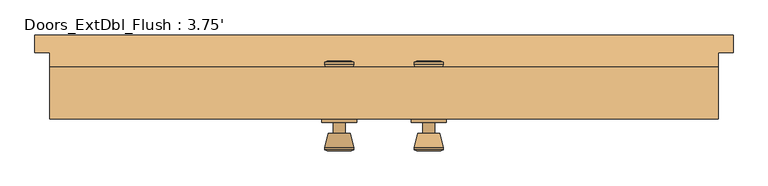
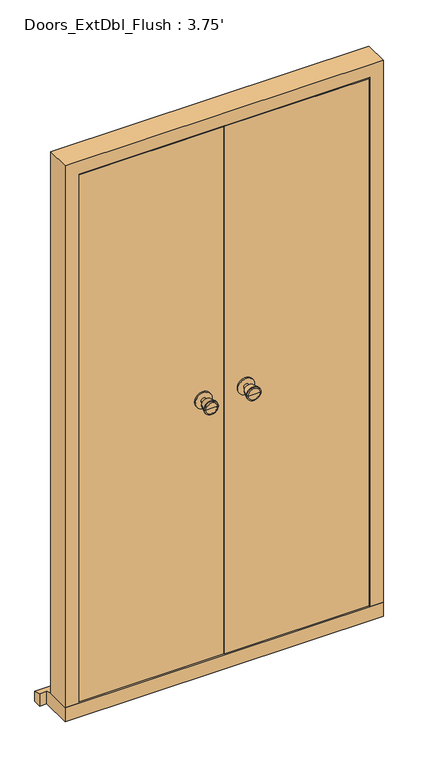
"""IFC4 building model written with IfcOpenShell, lengths in millimetres: door geometry, Doors_ExtDbl_Flush : 3.75'."""

from ifc_helpers import new_model, si_unit, point, frame, frame_2d, origin, place, context, project, spatial, polyline, circle_curve, trimmed, segment, composite_curve, outline, extrude, faceted_brep, source, transform, mapped, element, save
from ifc_brep_helpers import plane_surface, cylinder_surface, revolved_surface, advanced_brep


def doors_extdbl_flush_3_75_39ca422f(model_context):
    return source(origin(), model_context, "Body", "SolidModel", [
        advanced_brep(
        [(-76.5, -43.8, 1050.0), (-66.5, -43.8, 1050.0), (-86.5, -43.8, 1050.0), (-96.9758676, -92.8, 1050.0), (-56.0241324, -92.8, 1050.0), (-76.5, -92.8, 1050.0), (-101.5, -90.9721319, 1050.0), (-51.5, -90.9721319, 1050.0), (-101.5, -87.5084537, 1050.0), (-51.5, -87.5084537, 1050.0), (-95.136236, -62.8, 1050.0), (-57.863764, -62.8, 1050.0), (-86.5, -62.8, 1050.0), (-66.5, -62.8, 1050.0)],
        [
            (0, 1),
            (1, 2, circle_curve(frame((-76.5, -43.8, 1050.0), z_axis=(0.0, 1.0, 0.0), x_axis=(1.0, 0.0, 0.0)), 10.0)),
            (2, 0),
            (2, 1, circle_curve(frame((-76.5, -43.8, 1050.0), z_axis=(0.0, 1.0, 0.0), x_axis=(1.0, 0.0, 0.0)), 10.0)),
            (3, 4, circle_curve(frame((-76.5, -92.8, 1050.0), z_axis=(0.0, -1.0, 0.0), x_axis=(1.0, 0.0, 0.0)), 20.4758676)),
            (4, 5),
            (5, 3),
            (4, 3, circle_curve(frame((-76.5, -92.8, 1050.0), z_axis=(0.0, -1.0, 0.0), x_axis=(1.0, 0.0, 0.0)), 20.4758676)),
            (6, 7, circle_curve(frame((-76.5, -90.9721319, 1050.0), z_axis=(0.0, -1.0, 0.0), x_axis=(1.0, 0.0, 0.0)), 25.0)),
            (7, 4),
            (3, 6),
            (7, 6, circle_curve(frame((-76.5, -90.9721319, 1050.0), z_axis=(0.0, -1.0, 0.0), x_axis=(1.0, 0.0, 0.0)), 25.0)),
            (8, 9, circle_curve(frame((-76.5, -87.5084537, 1050.0), z_axis=(0.0, -1.0, 0.0), x_axis=(1.0, 0.0, 0.0)), 25.0)),
            (9, 7),
            (6, 8),
            (9, 8, circle_curve(frame((-76.5, -87.5084537, 1050.0), z_axis=(0.0, -1.0, 0.0), x_axis=(1.0, 0.0, 0.0)), 25.0)),
            (10, 11, circle_curve(frame((-76.5, -62.8, 1050.0), z_axis=(0.0, -1.0, 0.0), x_axis=(1.0, 0.0, 0.0)), 18.636236)),
            (11, 9),
            (8, 10),
            (11, 10, circle_curve(frame((-76.5, -62.8, 1050.0), z_axis=(0.0, -1.0, 0.0), x_axis=(1.0, 0.0, 0.0)), 18.636236)),
            (12, 13, circle_curve(frame((-76.5, -62.8, 1050.0), z_axis=(0.0, -1.0, 0.0), x_axis=(1.0, 0.0, 0.0)), 10.0)),
            (13, 11),
            (10, 12),
            (13, 12, circle_curve(frame((-76.5, -62.8, 1050.0), z_axis=(0.0, -1.0, 0.0), x_axis=(1.0, 0.0, 0.0)), 10.0)),
            (1, 13),
            (12, 2),
        ],
        [
            plane_surface(frame((-76.5, -43.8, 1050.0), z_axis=(0.0, 1.0, 0.0), x_axis=(1.0, 0.0, 0.0))),
            plane_surface(frame((-76.5, -92.8, 1050.0), z_axis=(0.0, -1.0, 0.0), x_axis=(1.0, 0.0, 0.0))),
            revolved_surface(polyline([(-56.0241324, -92.8, 1050.0), (-51.5, -90.9721319, 1050.0)]), (-76.5, -43.8, 1050.0), (0.0, 1.0, 0.0)),
            cylinder_surface(frame((-76.5, -43.8, 1050.0), z_axis=(0.0, 1.0, 0.0), x_axis=(1.0, 0.0, 0.0)), 25.0),
            revolved_surface(polyline([(-51.5, -87.5084537, 1050.0), (-57.863764, -62.8, 1050.0)]), (-76.5, -43.8, 1050.0), (0.0, 1.0, 0.0)),
            plane_surface(frame((-76.5, -62.8, 1050.0), z_axis=(0.0, 1.0, 0.0), x_axis=(1.0, 0.0, 0.0))),
            cylinder_surface(frame((-76.5, -43.8, 1050.0), z_axis=(0.0, 1.0, 0.0), x_axis=(1.0, 0.0, 0.0)), 10.0),
        ],
        [
            (0, [[1, 2, 3]]),
            (0, [[-3, 4, -1]]),
            (1, [[5, 6, 7]]),
            (1, [[8, -7, -6]]),
            (2, [[9, 10, -5, 11]]),
            (2, [[12, -11, -8, -10]]),
            (3, [[13, 14, -9, 15]]),
            (3, [[16, -15, -12, -14]]),
            (4, [[17, 18, -13, 19]]),
            (4, [[20, -19, -16, -18]]),
            (5, [[21, 22, -17, 23]]),
            (5, [[24, -23, -20, -22]]),
            (6, [[-2, 25, -21, 26]]),
            (6, [[-4, -26, -24, -25]]),
        ],
    ),
        extrude(outline(composite_curve([segment(trimmed(circle_curve(frame_2d((1050.0, -76.5)), 30.0), [point((1050.0, -46.5))], [point((1050.0, -106.5))], False, "CARTESIAN"), True, "CONTINUOUS"), segment(trimmed(circle_curve(frame_2d((1050.0, -76.5)), 30.0), [point((1050.0, -106.5))], [point((1050.0, -46.5))], False, "CARTESIAN"), True, "CONTINUOUS")], self_intersect=False)), frame((0.0, -43.8, 0.0), z_axis=(0.0, 1.0, 0.0), x_axis=(0.0, 0.0, 1.0)), (0.0, 0.0, 1.0), 6.0),
        advanced_brep(
        [(-76.5, 12.2, 1050.0), (-86.5, 12.2, 1050.0), (-66.5, 12.2, 1050.0), (-96.9758676, 61.2, 1050.0), (-76.5, 61.2, 1050.0), (-56.0241324, 61.2, 1050.0), (-101.5, 59.3721319, 1050.0), (-51.5, 59.3721319, 1050.0), (-101.5, 55.9084537, 1050.0), (-51.5, 55.9084537, 1050.0), (-95.136236, 31.2, 1050.0), (-57.863764, 31.2, 1050.0), (-86.5, 31.2, 1050.0), (-66.5, 31.2, 1050.0)],
        [
            (0, 1),
            (1, 2, circle_curve(frame((-76.5, 12.2, 1050.0), z_axis=(0.0, -1.0, 0.0), x_axis=(1.0, 0.0, 0.0)), 10.0)),
            (2, 0),
            (2, 1, circle_curve(frame((-76.5, 12.2, 1050.0), z_axis=(0.0, -1.0, 0.0), x_axis=(1.0, 0.0, 0.0)), 10.0)),
            (3, 4),
            (4, 5),
            (5, 3, circle_curve(frame((-76.5, 61.2, 1050.0), z_axis=(0.0, 1.0, 0.0), x_axis=(1.0, 0.0, 0.0)), 20.4758676)),
            (3, 5, circle_curve(frame((-76.5, 61.2, 1050.0), z_axis=(0.0, 1.0, 0.0), x_axis=(1.0, 0.0, 0.0)), 20.4758676)),
            (6, 3),
            (5, 7),
            (7, 6, circle_curve(frame((-76.5, 59.3721319, 1050.0), z_axis=(0.0, 1.0, 0.0), x_axis=(1.0, 0.0, 0.0)), 25.0)),
            (6, 7, circle_curve(frame((-76.5, 59.3721319, 1050.0), z_axis=(0.0, 1.0, 0.0), x_axis=(1.0, 0.0, 0.0)), 25.0)),
            (8, 6),
            (7, 9),
            (9, 8, circle_curve(frame((-76.5, 55.9084537, 1050.0), z_axis=(0.0, 1.0, 0.0), x_axis=(1.0, 0.0, 0.0)), 25.0)),
            (8, 9, circle_curve(frame((-76.5, 55.9084537, 1050.0), z_axis=(0.0, 1.0, 0.0), x_axis=(1.0, 0.0, 0.0)), 25.0)),
            (10, 8),
            (9, 11),
            (11, 10, circle_curve(frame((-76.5, 31.2, 1050.0), z_axis=(0.0, 1.0, 0.0), x_axis=(1.0, 0.0, 0.0)), 18.636236)),
            (10, 11, circle_curve(frame((-76.5, 31.2, 1050.0), z_axis=(0.0, 1.0, 0.0), x_axis=(1.0, 0.0, 0.0)), 18.636236)),
            (12, 10),
            (11, 13),
            (13, 12, circle_curve(frame((-76.5, 31.2, 1050.0), z_axis=(0.0, 1.0, 0.0), x_axis=(1.0, 0.0, 0.0)), 10.0)),
            (12, 13, circle_curve(frame((-76.5, 31.2, 1050.0), z_axis=(0.0, 1.0, 0.0), x_axis=(1.0, 0.0, 0.0)), 10.0)),
            (1, 12),
            (13, 2),
        ],
        [
            plane_surface(frame((-76.5, 12.2, 1050.0), z_axis=(0.0, -1.0, 0.0), x_axis=(1.0, 0.0, 0.0))),
            plane_surface(frame((-76.5, 61.2, 1050.0), z_axis=(0.0, 1.0, 0.0), x_axis=(1.0, 0.0, 0.0))),
            revolved_surface(polyline([(-56.0241324, 61.2, 1050.0), (-51.5, 59.3721319, 1050.0)]), (-76.5, 12.2, 1050.0), (0.0, -1.0, 0.0)),
            cylinder_surface(frame((-76.5, 12.2, 1050.0), z_axis=(0.0, -1.0, 0.0), x_axis=(1.0, 0.0, 0.0)), 25.0),
            revolved_surface(polyline([(-51.5, 55.9084537, 1050.0), (-57.863764, 31.2, 1050.0)]), (-76.5, 12.2, 1050.0), (0.0, -1.0, 0.0)),
            plane_surface(frame((-76.5, 31.2, 1050.0), z_axis=(0.0, -1.0, 0.0), x_axis=(1.0, 0.0, 0.0))),
            cylinder_surface(frame((-76.5, 12.2, 1050.0), z_axis=(0.0, -1.0, 0.0), x_axis=(1.0, 0.0, 0.0)), 10.0),
        ],
        [
            (0, [[1, 2, 3]]),
            (0, [[-3, 4, -1]]),
            (1, [[5, 6, 7]]),
            (1, [[-6, -5, 8]]),
            (2, [[9, -7, 10, 11]]),
            (2, [[-10, -8, -9, 12]]),
            (3, [[13, -11, 14, 15]]),
            (3, [[-14, -12, -13, 16]]),
            (4, [[17, -15, 18, 19]]),
            (4, [[-18, -16, -17, 20]]),
            (5, [[21, -19, 22, 23]]),
            (5, [[-22, -20, -21, 24]]),
            (6, [[25, -23, 26, -2]]),
            (6, [[-26, -24, -25, -4]]),
        ],
    ),
        extrude(outline(composite_curve([segment(trimmed(circle_curve(frame_2d((1050.0, -76.5)), 30.0), [point((1050.0, -46.5))], [point((1050.0, -106.5))], False, "CARTESIAN"), True, "CONTINUOUS"), segment(trimmed(circle_curve(frame_2d((1050.0, -76.5)), 30.0), [point((1050.0, -106.5))], [point((1050.0, -46.5))], False, "CARTESIAN"), True, "CONTINUOUS")], self_intersect=False)), frame((0.0, 6.2, 0.0), z_axis=(0.0, 1.0, 0.0), x_axis=(0.0, 0.0, 1.0)), (0.0, 0.0, 1.0), 6.0),
        advanced_brep(
        [(76.5, -43.8, 1050.0), (86.5, -43.8, 1050.0), (66.5, -43.8, 1050.0), (96.9758676, -92.8, 1050.0), (76.5, -92.8, 1050.0), (56.0241324, -92.8, 1050.0), (101.5, -90.9721319, 1050.0), (51.5, -90.9721319, 1050.0), (101.5, -87.5084537, 1050.0), (51.5, -87.5084537, 1050.0), (95.136236, -62.8, 1050.0), (57.863764, -62.8, 1050.0), (86.5, -62.8, 1050.0), (66.5, -62.8, 1050.0)],
        [
            (0, 1),
            (1, 2, circle_curve(frame((76.5, -43.8, 1050.0), z_axis=(0.0, 1.0, 0.0), x_axis=(-1.0, 0.0, 0.0)), 10.0)),
            (2, 0),
            (2, 1, circle_curve(frame((76.5, -43.8, 1050.0), z_axis=(0.0, 1.0, 0.0), x_axis=(-1.0, 0.0, 0.0)), 10.0)),
            (3, 4),
            (4, 5),
            (5, 3, circle_curve(frame((76.5, -92.8, 1050.0), z_axis=(0.0, -1.0, 0.0), x_axis=(-1.0, 0.0, 0.0)), 20.4758676)),
            (3, 5, circle_curve(frame((76.5, -92.8, 1050.0), z_axis=(0.0, -1.0, 0.0), x_axis=(-1.0, 0.0, 0.0)), 20.4758676)),
            (6, 3),
            (5, 7),
            (7, 6, circle_curve(frame((76.5, -90.9721319, 1050.0), z_axis=(0.0, -1.0, 0.0), x_axis=(-1.0, 0.0, 0.0)), 25.0)),
            (6, 7, circle_curve(frame((76.5, -90.9721319, 1050.0), z_axis=(0.0, -1.0, 0.0), x_axis=(-1.0, 0.0, 0.0)), 25.0)),
            (8, 6),
            (7, 9),
            (9, 8, circle_curve(frame((76.5, -87.5084537, 1050.0), z_axis=(0.0, -1.0, 0.0), x_axis=(-1.0, 0.0, 0.0)), 25.0)),
            (8, 9, circle_curve(frame((76.5, -87.5084537, 1050.0), z_axis=(0.0, -1.0, 0.0), x_axis=(-1.0, 0.0, 0.0)), 25.0)),
            (10, 8),
            (9, 11),
            (11, 10, circle_curve(frame((76.5, -62.8, 1050.0), z_axis=(0.0, -1.0, 0.0), x_axis=(-1.0, 0.0, 0.0)), 18.636236)),
            (10, 11, circle_curve(frame((76.5, -62.8, 1050.0), z_axis=(0.0, -1.0, 0.0), x_axis=(-1.0, 0.0, 0.0)), 18.636236)),
            (12, 10),
            (11, 13),
            (13, 12, circle_curve(frame((76.5, -62.8, 1050.0), z_axis=(0.0, -1.0, 0.0), x_axis=(-1.0, 0.0, 0.0)), 10.0)),
            (12, 13, circle_curve(frame((76.5, -62.8, 1050.0), z_axis=(0.0, -1.0, 0.0), x_axis=(-1.0, 0.0, 0.0)), 10.0)),
            (1, 12),
            (13, 2),
        ],
        [
            plane_surface(frame((76.5, -43.8, 1050.0), z_axis=(0.0, 1.0, 0.0), x_axis=(-1.0, 0.0, 0.0))),
            plane_surface(frame((76.5, -92.8, 1050.0), z_axis=(0.0, -1.0, 0.0), x_axis=(-1.0, 0.0, 0.0))),
            revolved_surface(polyline([(56.0241324, -92.8, 1050.0), (51.5, -90.9721319, 1050.0)]), (76.5, -43.8, 1050.0), (0.0, 1.0, 0.0)),
            cylinder_surface(frame((76.5, -43.8, 1050.0), z_axis=(0.0, 1.0, 0.0), x_axis=(-1.0, 0.0, 0.0)), 25.0),
            revolved_surface(polyline([(51.5, -87.5084537, 1050.0), (57.863764, -62.8, 1050.0)]), (76.5, -43.8, 1050.0), (0.0, 1.0, 0.0)),
            plane_surface(frame((76.5, -62.8, 1050.0), z_axis=(0.0, 1.0, 0.0), x_axis=(-1.0, 0.0, 0.0))),
            cylinder_surface(frame((76.5, -43.8, 1050.0), z_axis=(0.0, 1.0, 0.0), x_axis=(-1.0, 0.0, 0.0)), 10.0),
        ],
        [
            (0, [[1, 2, 3]]),
            (0, [[-3, 4, -1]]),
            (1, [[5, 6, 7]]),
            (1, [[-6, -5, 8]]),
            (2, [[9, -7, 10, 11]]),
            (2, [[-10, -8, -9, 12]]),
            (3, [[13, -11, 14, 15]]),
            (3, [[-14, -12, -13, 16]]),
            (4, [[17, -15, 18, 19]]),
            (4, [[-18, -16, -17, 20]]),
            (5, [[21, -19, 22, 23]]),
            (5, [[-22, -20, -21, 24]]),
            (6, [[25, -23, 26, -2]]),
            (6, [[-26, -24, -25, -4]]),
        ],
    ),
        extrude(outline(composite_curve([segment(trimmed(circle_curve(frame_2d((1050.0, 76.5)), 30.0), [point((1050.0, 46.5))], [point((1050.0, 106.5))], False, "CARTESIAN"), True, "CONTINUOUS"), segment(trimmed(circle_curve(frame_2d((1050.0, 76.5)), 30.0), [point((1050.0, 106.5))], [point((1050.0, 46.5))], False, "CARTESIAN"), True, "CONTINUOUS")], self_intersect=False)), frame((0.0, -43.8, 0.0), z_axis=(0.0, 1.0, 0.0), x_axis=(0.0, 0.0, 1.0)), (0.0, 0.0, 1.0), 6.0),
        advanced_brep(
        [(76.5, 12.2, 1050.0), (66.5, 12.2, 1050.0), (86.5, 12.2, 1050.0), (96.9758676, 61.2, 1050.0), (56.0241324, 61.2, 1050.0), (76.5, 61.2, 1050.0), (101.5, 59.3721319, 1050.0), (51.5, 59.3721319, 1050.0), (101.5, 55.9084537, 1050.0), (51.5, 55.9084537, 1050.0), (95.136236, 31.2, 1050.0), (57.863764, 31.2, 1050.0), (86.5, 31.2, 1050.0), (66.5, 31.2, 1050.0)],
        [
            (0, 1),
            (1, 2, circle_curve(frame((76.5, 12.2, 1050.0), z_axis=(0.0, -1.0, 0.0), x_axis=(-1.0, 0.0, 0.0)), 10.0)),
            (2, 0),
            (2, 1, circle_curve(frame((76.5, 12.2, 1050.0), z_axis=(0.0, -1.0, 0.0), x_axis=(-1.0, 0.0, 0.0)), 10.0)),
            (3, 4, circle_curve(frame((76.5, 61.2, 1050.0), z_axis=(0.0, 1.0, 0.0), x_axis=(-1.0, 0.0, 0.0)), 20.4758676)),
            (4, 5),
            (5, 3),
            (4, 3, circle_curve(frame((76.5, 61.2, 1050.0), z_axis=(0.0, 1.0, 0.0), x_axis=(-1.0, 0.0, 0.0)), 20.4758676)),
            (6, 7, circle_curve(frame((76.5, 59.3721319, 1050.0), z_axis=(0.0, 1.0, 0.0), x_axis=(-1.0, 0.0, 0.0)), 25.0)),
            (7, 4),
            (3, 6),
            (7, 6, circle_curve(frame((76.5, 59.3721319, 1050.0), z_axis=(0.0, 1.0, 0.0), x_axis=(-1.0, 0.0, 0.0)), 25.0)),
            (8, 9, circle_curve(frame((76.5, 55.9084537, 1050.0), z_axis=(0.0, 1.0, 0.0), x_axis=(-1.0, 0.0, 0.0)), 25.0)),
            (9, 7),
            (6, 8),
            (9, 8, circle_curve(frame((76.5, 55.9084537, 1050.0), z_axis=(0.0, 1.0, 0.0), x_axis=(-1.0, 0.0, 0.0)), 25.0)),
            (10, 11, circle_curve(frame((76.5, 31.2, 1050.0), z_axis=(0.0, 1.0, 0.0), x_axis=(-1.0, 0.0, 0.0)), 18.636236)),
            (11, 9),
            (8, 10),
            (11, 10, circle_curve(frame((76.5, 31.2, 1050.0), z_axis=(0.0, 1.0, 0.0), x_axis=(-1.0, 0.0, 0.0)), 18.636236)),
            (12, 13, circle_curve(frame((76.5, 31.2, 1050.0), z_axis=(0.0, 1.0, 0.0), x_axis=(-1.0, 0.0, 0.0)), 10.0)),
            (13, 11),
            (10, 12),
            (13, 12, circle_curve(frame((76.5, 31.2, 1050.0), z_axis=(0.0, 1.0, 0.0), x_axis=(-1.0, 0.0, 0.0)), 10.0)),
            (1, 13),
            (12, 2),
        ],
        [
            plane_surface(frame((76.5, 12.2, 1050.0), z_axis=(0.0, -1.0, 0.0), x_axis=(-1.0, 0.0, 0.0))),
            plane_surface(frame((76.5, 61.2, 1050.0), z_axis=(0.0, 1.0, 0.0), x_axis=(-1.0, 0.0, 0.0))),
            revolved_surface(polyline([(56.0241324, 61.2, 1050.0), (51.5, 59.3721319, 1050.0)]), (76.5, 12.2, 1050.0), (0.0, -1.0, 0.0)),
            cylinder_surface(frame((76.5, 12.2, 1050.0), z_axis=(0.0, -1.0, 0.0), x_axis=(-1.0, 0.0, 0.0)), 25.0),
            revolved_surface(polyline([(51.5, 55.9084537, 1050.0), (57.863764, 31.2, 1050.0)]), (76.5, 12.2, 1050.0), (0.0, -1.0, 0.0)),
            plane_surface(frame((76.5, 31.2, 1050.0), z_axis=(0.0, -1.0, 0.0), x_axis=(-1.0, 0.0, 0.0))),
            cylinder_surface(frame((76.5, 12.2, 1050.0), z_axis=(0.0, -1.0, 0.0), x_axis=(-1.0, 0.0, 0.0)), 10.0),
        ],
        [
            (0, [[1, 2, 3]]),
            (0, [[-3, 4, -1]]),
            (1, [[5, 6, 7]]),
            (1, [[8, -7, -6]]),
            (2, [[9, 10, -5, 11]]),
            (2, [[12, -11, -8, -10]]),
            (3, [[13, 14, -9, 15]]),
            (3, [[16, -15, -12, -14]]),
            (4, [[17, 18, -13, 19]]),
            (4, [[20, -19, -16, -18]]),
            (5, [[21, 22, -17, 23]]),
            (5, [[24, -23, -20, -22]]),
            (6, [[-2, 25, -21, 26]]),
            (6, [[-4, -26, -24, -25]]),
        ],
    ),
        extrude(outline(composite_curve([segment(trimmed(circle_curve(frame_2d((1050.0, 76.5)), 30.0), [point((1050.0, 46.5))], [point((1050.0, 106.5))], False, "CARTESIAN"), True, "CONTINUOUS"), segment(trimmed(circle_curve(frame_2d((1050.0, 76.5)), 30.0), [point((1050.0, 106.5))], [point((1050.0, 46.5))], False, "CARTESIAN"), True, "CONTINUOUS")], self_intersect=False)), frame((0.0, 6.2, 0.0), z_axis=(0.0, 1.0, 0.0), x_axis=(0.0, 0.0, 1.0)), (0.0, 0.0, 1.0), 6.0),
        faceted_brep([(501.0, 51.2, 54.5), (571.5, 51.2, 54.5), (571.5, -37.8, 54.5), (523.0, -37.8, 54.5), (523.0, 9.2, 54.5), (501.0, 9.2, 54.5), (501.0, 51.2, 2039.5), (-501.0, 51.2, 2039.5), (-501.0, 51.2, 54.5), (-571.5, 51.2, 54.5), (-571.5, 51.2, 2110.0), (571.5, 51.2, 2110.0), (571.5, -37.8, 2110.0), (-571.5, -37.8, 2110.0), (-571.5, -37.8, 54.5), (-523.0, -37.8, 54.5), (-523.0, -37.8, 2061.5), (523.0, -37.8, 2061.5), (523.0, 9.2, 2061.5), (-523.0, 9.2, 2061.5), (-523.0, 9.2, 54.5), (-501.0, 9.2, 54.5), (-501.0, 9.2, 2039.5), (501.0, 9.2, 2039.5)], [[[0, 1, 2, 3, 4, 5]], [[1, 0, 6, 7, 8, 9, 10, 11]], [[2, 1, 11, 12]], [[3, 2, 12, 13, 14, 15, 16, 17]], [[4, 3, 17, 18]], [[5, 4, 18, 19, 20, 21, 22, 23]], [[0, 5, 23, 6]], [[7, 22, 21, 8]], [[8, 21, 20, 15, 14, 9]], [[13, 10, 9, 14]], [[19, 16, 15, 20]], [[12, 11, 10, 13]], [[18, 17, 16, 19]], [[6, 23, 22, 7]]]),
        faceted_brep([(596.5, 106.2, 0.0), (596.5, 106.2, 38.5947221), (596.5, 76.2, 47.2703282), (596.5, 76.2, 0.0), (-596.5, 106.2, 38.5947221), (-596.5, 106.2, 0.0), (-596.5, 76.2, 0.0), (-596.5, 76.2, 47.2703282), (571.5, 76.2, 0.0), (571.5, -37.8, 0.0), (-571.5, -37.8, 0.0), (-571.5, 76.2, 0.0), (-571.5, 76.2, 47.2703282), (-571.5, 51.2, 54.5), (571.5, 51.2, 54.5), (571.5, 76.2, 47.2703282), (-571.5, -37.8, 54.5), (571.5, -37.8, 54.5)], [[[0, 1, 2, 3]], [[4, 5, 6, 7]], [[5, 0, 3, 8, 9, 10, 11, 6]], [[1, 0, 5, 4]], [[1, 4, 7, 12, 13, 14, 15, 2]], [[13, 16, 17, 14]], [[16, 10, 9, 17]], [[12, 11, 10, 16, 13]], [[11, 12, 7, 6]], [[8, 15, 14, 17, 9]], [[15, 8, 3, 2]]]),
        extrude(outline(polyline([(520.0, -37.8), (1.5, -37.8), (1.5, 6.2), (520.0, 6.2), (520.0, -37.8)])), frame((0.0, 0.0, 58.5), z_axis=(0.0, 0.0, 1.0), x_axis=(1.0, 0.0, 0.0)), (0.0, 0.0, 1.0), 2000.0),
        extrude(outline(polyline([(-1.5, -37.8), (-520.0, -37.8), (-520.0, 6.2), (-1.5, 6.2), (-1.5, -37.8)])), frame((0.0, 0.0, 58.5), z_axis=(0.0, 0.0, 1.0), x_axis=(1.0, 0.0, 0.0)), (0.0, 0.0, 1.0), 2000.0),
    ])


if __name__ == "__main__":
    model = new_model("IFC4")
    model_context = context("Model", 3, world=origin())
    ifc_project = project(units=[si_unit("LENGTHUNIT", "METRE", prefix="MILLI")], contexts=[model_context])
    site = spatial("IfcSite", under=ifc_project)
    building = spatial("IfcBuilding", under=site)
    placement = place(None, origin())
    doors_extdbl_flush_3_75_shape = doors_extdbl_flush_3_75_39ca422f(model_context)
    element("IfcDoor", 1, ObjectType="Doors_ExtDbl_Flush : 3.75'", at=placement, inside=building, context=model_context, shape_type="MappedRepresentation", body=[
        mapped(doors_extdbl_flush_3_75_shape, transform((0.0, 0.0, 0.0), x_axis=(1.0, 0.0, 0.0), y_axis=(0.0, 1.0, 0.0), z_axis=(0.0, 0.0, 1.0))),
    ])
    save(model, "model.ifc")

# Revit data of these elements
# Type "Doors_ExtDbl_Flush : 3.75'"
#   Type Mark = "54"
#   Type Comments = "External Double"
#   Operation = "DoubleDoorSingleSwing"
#   Keynote = "L20"
#   Analytic Construction = "Metal"
#   Wrap Layers (Ext) from Ext = 102.5 mm
#   Wrap Layers (Int) from Ext = 177.5 mm
#   Thickness = 44 mm
#   Rough Width = 1143 mm
#   Rough Height = 2110 mm
#   O/A Frame Width = 64 mm
#   Heat Transfer Coefficient (U) = 3.7021 W/(m²·K)
#   Handle Z Distance = 1050 mm
#   FrameWidth = 42 mm
#   FrameOffset - External = 25 mm
#   FrameDepth = 89 mm
#   Door Panel Width = 518.5 mm
#   Door Panel Thickness = 44 mm
#   Door Panel Height = 2000 mm
#   Cill Thickness = 54.5 mm
#   Cill Projection = 30 mm
#   Handle X Distance = 75 mm
#   Height = 2110 mm
#   Structural Tolerance = 6.5 mm
#   Tolerance = 3 mm
#   Undercut = 4 mm
#   Width = 1143 mm
#   Cill Extension = 25 mm
#   Cavity Closer Width = 50 mm
#   Cavity Closer Offset from Ext = 102.5 mm
#   Cavity Closer Depth = 85 mm
#   Vis - Ironmongery = yes
#   Vis - Cavity Closers = yes
#   Function = 1
#   Material Door = Door - Panel
#   Material Frame = Door - Frame/Mullion
#   Material Ironmongery = Door - Handle
#   Visual Light Transmittance = 0
#   Thermal Resistance (R) = 0
#   Solar Heat Gain Coefficient = 0
#   Wall Closure = (empty or 0)
# Element 1 (IfcDoor, "Doors_ExtDbl_Flush : 3.75'")
#   Materials on its faces: "Door - Handle", "Door - Frame/Mullion", "Door - Panel"
# Materials
#   "Door - Panel": class "Wood", colour RGB 210 159 95, transparency 0, Keynote = "L20", Cost = 0
#   "Door - Frame/Mullion": class "Wood", colour RGB 212 179 113, transparency 0, Keynote = "L20", Cost = 0
#   "Door - Handle": colour RGB 0 0 0, transparency 0, Keynote = "P21", Cost = 0
